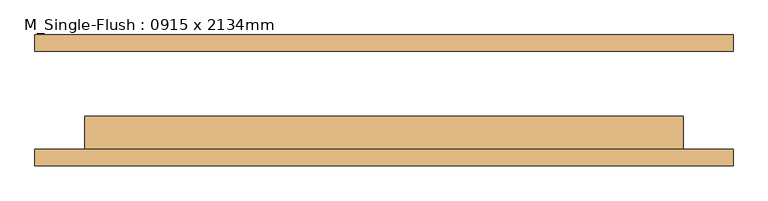
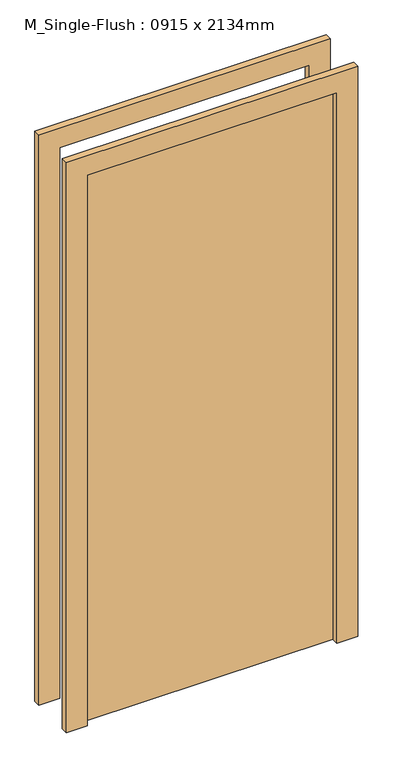
"""IFC4 building model written with IfcOpenShell, lengths in millimetres: door geometry, M_Single-Flush : 0915 x 2134mm."""

from ifc_helpers import new_model, si_unit, frame, origin, origin_with_axes, place, context, project, spatial, polyline, outline, extrude, source, transform, mapped, element, save


def m_single_flush_0915_x_2134mm_f3d7f739(model_context):
    return source(origin(), model_context, "Body", "SweptSolid", [
        extrude(outline(polyline([(2210.0, -533.5), (0.0, -533.5), (0.0, -457.5), (2134.0, -457.5), (2134.0, 457.5), (0.0, 457.5), (0.0, 533.5), (2210.0, 533.5), (2210.0, -533.5)])), frame((0.0, -100.0, 0.0), z_axis=(0.0, 1.0, 0.0), x_axis=(0.0, 0.0, 1.0)), (0.0, 0.0, 1.0), 25.0),
        extrude(outline(polyline([(2210.0, 533.5), (2210.0, -533.5), (0.0, -533.5), (0.0, -457.5), (2134.0, -457.5), (2134.0, 457.5), (0.0, 457.5), (0.0, 533.5), (2210.0, 533.5)])), frame((0.0, 75.0, 0.0), z_axis=(0.0, 1.0, 0.0), x_axis=(0.0, 0.0, 1.0)), (0.0, 0.0, 1.0), 25.0),
        extrude(outline(polyline([(457.5, -24.0), (457.5, -75.0), (-457.5, -75.0), (-457.5, -24.0), (457.5, -24.0)])), origin_with_axes(), (0.0, 0.0, 1.0), 2134.0),
    ])


if __name__ == "__main__":
    model = new_model("IFC4")
    model_context = context("Model", 3, world=origin())
    ifc_project = project(units=[si_unit("LENGTHUNIT", "METRE", prefix="MILLI")], contexts=[model_context])
    site = spatial("IfcSite", under=ifc_project)
    building = spatial("IfcBuilding", under=site)
    placement = place(None, origin())
    m_single_flush_0915_x_2134mm_shape = m_single_flush_0915_x_2134mm_f3d7f739(model_context)
    element("IfcDoor", 1, ObjectType="M_Single-Flush : 0915 x 2134mm", at=placement, inside=building, context=model_context, shape_type="MappedRepresentation", body=[
        mapped(m_single_flush_0915_x_2134mm_shape, transform((0.0, 0.0, 0.0), x_axis=(1.0, 0.0, 0.0), y_axis=(0.0, 1.0, 0.0), z_axis=(0.0, 0.0, 1.0))),
    ])
    save(model, "model.ifc")

# Revit data of these elements
# Type "M_Single-Flush : 0915 x 2134mm"
#   Type Mark = "15"
#   Thickness = 51 mm
#   Height = 2134 mm
#   Trim Projection Ext = 25 mm
#   Trim Projection Int = 25 mm
#   Trim Width = 76 mm
#   Width = 915 mm
#   Door Material = Door - Panel
#   Frame Material = Door - Frame
#   Function = (empty or 0)
#   Wall Closure = (empty or 0)
# Element 1 (IfcDoor, "M_Single-Flush : 0915 x 2134mm")
#   Materials on its faces: "Door - Frame", "Door - Panel"
# Materials
#   "Door - Panel": class "Wood", colour RGB 114 82 51, transparency 0
#   "Door - Frame": colour RGB 153 76 43, transparency 0
